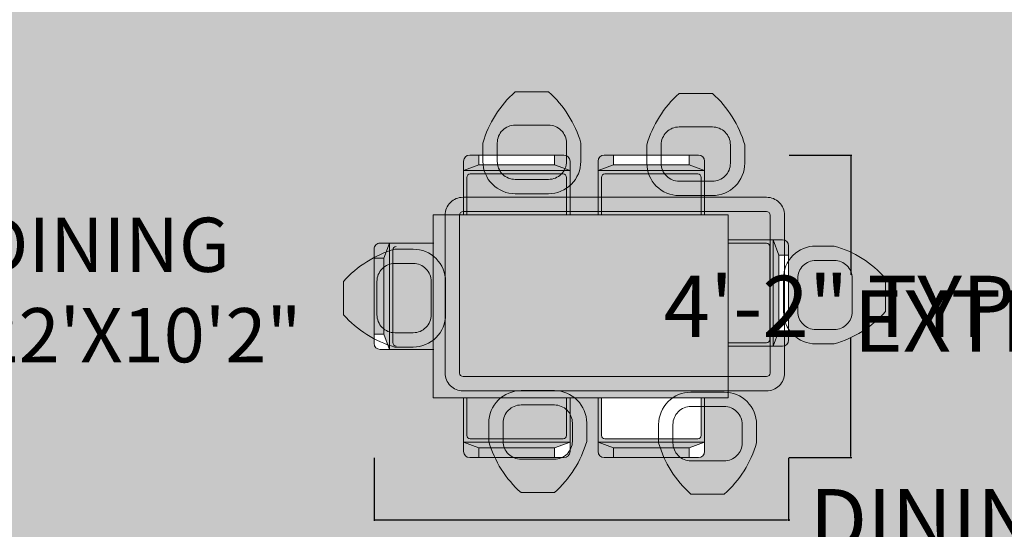
# Model space of a CAD drawing. Units: inches. Extents: x 1077 to 2505, y 1892 to 2728.
# Tile 14 of 26: x 1306 to 1470, y 2338 to 2422. Entities that reach past the tile are written whole.
import ezdxf

# ---------------------------------------------------------------- set-up
doc = ezdxf.new("R2010")
doc.units = ezdxf.units.IN
doc.linetypes.add('ACAD_ISO02W100', pattern=[15, 12, -3])
doc.layers.get('Defpoints').update_dxf_attribs({"color": 220, "linetype": 'ACAD_ISO02W100'})
for name, color, linetype, lineweight in [('00 FURNITURE', 15, 'Continuous', 15), ('A-ANNO-DIMS', 2, 'Continuous', 18), ('A-AREA-IDEN', 7, 'Continuous', 18)]:
    doc.layers.add(name, color=color, linetype=linetype, lineweight=lineweight)
doc.layers.add('A-FLOR-PATT', color=254, linetype='Continuous', lineweight=9, true_color=0xd7ebd2)
doc.styles.get("Standard").update_dxf_attribs({"font": 'arial.ttf'})
doc.dimstyles.get("Standard").update_dxf_attribs({"dimtxt": 10.18, "dimasz": 0.18, "dimexe": 0.18, "dimexo": 0.0625, "dimgap": 0.09, "dimtad": 0, "dimtih": 1, "dimtoh": 1, "dimdec": 0, "dimzin": 0, "dimdsep": 46, "dimlunit": 3, "dimtxsty": 'Standard', "dimcen": 0.09, "dimadec": 0, "dimazin": 0, "dimtfac": 1, "dimtdec": 0, "dimtofl": 0, "dimtmove": 0, "dimatfit": 3, "dimfxl": 1, "dimtolj": 1, "dimtzin": 0, "dimarcsym": 0})

# ---------------------------------------------------------------- blocks, each defined once
blk = doc.blocks.new('DINING-SET-6-SEAT')
for p, q in [((14.85, 40.27), (14.85, 49.18)), ((15.87, 50.2), (31.49, 50.2)), ((32.51, 49.18), (32.51, 40.27)), ((37.18, 40.27), (37.18, 49.18)), ((38.2, 50.2), (53.82, 50.2)), ((54.83, 49.18), (54.83, 40.27)), ((17.38, 48.59), (14.85, 47.63)), ((14.85, 47.63), (32.51, 47.63)), ((17.38, 48.59), (29.95, 48.59)), ((29.95, 48.59), (32.51, 47.63)), ((39.7, 48.59), (37.18, 47.63)), ((37.18, 47.63), (54.83, 47.63)), ((39.7, 48.59), (52.28, 48.59)), ((52.28, 48.59), (54.83, 47.63)), ((15.41, 40.27), (15.41, 46.51)), ((15.97, 47.07), (31.38, 47.07)), ((31.94, 46.51), (31.94, 40.27)), ((37.74, 40.27), (37.74, 46.51)), ((38.3, 47.07), (53.71, 47.07)), ((54.27, 46.51), (54.27, 40.27)), ((58.75, 40.27), (9.82, 40.27)), ((9.82, 9.93), (9.82, 40.27)), ((58.75, 9.93), (58.75, 40.27)), ((58.86, 36.15), (67.76, 36.15)), ((67.17, 33.62), (66.22, 36.15)), ((66.22, 36.15), (66.22, 18.49)), ((0, 34.59), (0, 18.97)), ((9.93, 35.61), (1.02, 35.61)), ((1.62, 33.08), (2.57, 35.61)), ((2.57, 35.61), (2.57, 17.96)), ((3.13, 34.49), (3.13, 19.08)), ((58.86, 35.58), (65.09, 35.58)), ((65.65, 35.02), (65.65, 19.61)), ((68.78, 35.13), (68.78, 19.51)), ((1.62, 33.08), (1.62, 20.51)), ((67.17, 33.62), (67.17, 21.04)), ((1.62, 20.51), (2.57, 17.96)), ((67.17, 21.04), (66.22, 18.49)), ((65.09, 19.05), (58.86, 19.05)), ((67.76, 18.49), (58.86, 18.49)), ((1.02, 17.96), (9.93, 17.96)), ((58.75, 9.93), (9.82, 9.93)), ((14.85, 9.93), (14.85, 1.02)), ((15.41, 9.93), (15.41, 3.69)), ((31.94, 3.69), (31.94, 9.93)), ((32.51, 1.02), (32.51, 9.93)), ((37.18, 9.93), (37.18, 1.02)), ((37.74, 9.93), (37.74, 3.69)), ((54.27, 3.69), (54.27, 9.93)), ((54.83, 1.02), (54.83, 9.93)), ((17.38, 1.61), (14.85, 2.57)), ((14.85, 2.57), (32.51, 2.57)), ((15.97, 3.13), (31.38, 3.13)), ((29.95, 1.61), (32.51, 2.57)), ((39.7, 1.61), (37.18, 2.57)), ((37.18, 2.57), (54.83, 2.57)), ((38.3, 3.13), (53.71, 3.13)), ((52.28, 1.61), (54.83, 2.57)), ((17.38, 1.61), (29.95, 1.61)), ((39.7, 1.61), (52.28, 1.61)), ((15.87, 0), (31.49, 0)), ((38.2, 0), (53.82, 0))]:
    blk.add_line(p, q)
for points in [[(17.38, 50.2), (29.95, 50.2), (29.95, 48.59), (17.38, 48.59)], [(39.7, 50.2), (52.28, 50.2), (52.28, 48.59), (39.7, 48.59)], [(0, 33.08), (0, 20.51), (1.62, 20.51), (1.62, 33.08)], [(68.78, 33.62), (68.78, 21.04), (67.17, 21.04), (67.17, 33.62)], [(17.38, 0), (29.95, 0), (29.95, 1.61), (17.38, 1.61)], [(39.7, 0), (52.28, 0), (52.28, 1.61), (39.7, 1.61)]]:
    blk.add_lwpolyline(points, close=True)
for centre, radius, start, end in [((15.87, 49.18), 1.02, 90.0001, 180.0001), ((31.49, 49.18), 1.02, 0.0001, 90.0001), ((38.2, 49.18), 1.02, 90.0001, 180.0001), ((53.82, 49.18), 1.02, 0.0001, 90.0001), ((15.97, 46.51), 0.56, 90.0001, 180.0001), ((31.38, 46.51), 0.56, 0.0001, 90.0001), ((38.3, 46.51), 0.56, 90.0001, 180.0001), ((53.71, 46.51), 0.56, 0.0001, 90.0001), ((67.76, 35.13), 1.02, 0.0001, 90.0001), ((1.02, 34.59), 1.02, 89.9999, 179.9999), ((3.69, 34.49), 0.56, 89.9999, 179.9999), ((65.09, 35.02), 0.56, 0.0001, 90.0001), ((65.09, 19.61), 0.56, 270.0001, 0.0001), ((1.02, 18.97), 1.02, 179.9999, 269.9999), ((3.69, 19.08), 0.56, 179.9999, 269.9999), ((67.76, 19.51), 1.02, 270.0001, 0.0001), ((15.97, 3.69), 0.56, 179.9999, 269.9999), ((31.38, 3.69), 0.56, 269.9999, 359.9999), ((38.3, 3.69), 0.56, 179.9999, 269.9999), ((53.71, 3.69), 0.56, 269.9999, 359.9999), ((15.87, 1.02), 1.02, 179.9999, 269.9999), ((31.49, 1.02), 1.02, 269.9999, 359.9999), ((38.2, 1.02), 1.02, 179.9999, 269.9999), ((53.82, 1.02), 1.02, 269.9999, 359.9999)]:
    blk.add_arc(centre, radius, start, end)
blk = doc.blocks.new('DINING-CHAIR')
for points in [[(5.36, 16.93), (10.88, 16.93, -0.142909), (16.24, 8.42), (16.24, 5.36, -0.414214), (10.88, 0), (5.36, 0, -0.414214), (0, 5.36), (0, 8.42, -0.142909)], [(5.36, 11.39), (10.88, 11.39, -0.414214), (13.86, 8.42), (13.86, 5.36, -0.414214), (10.88, 2.38), (5.36, 2.38, -0.414214), (2.38, 5.36), (2.38, 8.42, -0.414214)]]:
    blk.add_lwpolyline(points, format="xyb", close=True)
blk = doc.blocks.new('*D36')
at = {"layer": 'A-ANNO-DIMS', "color": 0, "lineweight": -2, "transparency": 16777216}
for p, q in [((1365.09, 2349.48), (1365.09, 2339.05)), ((1433.87, 2349.48), (1433.87, 2339.05)), ((1365.27, 2339.23), (1433.69, 2339.23)), ((1433.87, 2339.23), (1434.05, 2339.23))]:
    blk.add_line(p, q, dxfattribs=at)
at = {"layer": 'A-ANNO-DIMS', "color": 0, "transparency": 16777216}
for points in [[(1365.27, 2339.26), (1365.27, 2339.2), (1365.09, 2339.23)], [(1433.69, 2339.26), (1433.69, 2339.2), (1433.87, 2339.23)]]:
    blk.add_solid(points, dxfattribs=at)
at = {"layer": 'Defpoints', "color": 0, "transparency": 16777216}
for p in [(1365.09, 2349.54), (1433.87, 2349.54), (1433.87, 2339.23)]:
    blk.add_point(p, dxfattribs=at)
at = {"layer": 'A-ANNO-DIMS', "color": 0, "transparency": 16777216, "insert": (1507.58, 2339.23), "char_height": 10.18, "attachment_point": 5}
blk.add_mtext('\\A1;DINING SET 5\'-9" TYP.', dxfattribs=at)
blk = doc.blocks.new('*D37')
at = {"layer": 'A-ANNO-DIMS', "color": 0, "lineweight": -2, "transparency": 16777216}
for p, q in [((1433.94, 2399.74), (1444.37, 2399.74)), ((1444.19, 2399.56), (1444.19, 2379.85)), ((1444.19, 2349.72), (1444.19, 2369.44)), ((1433.94, 2349.54), (1444.37, 2349.54))]:
    blk.add_line(p, q, dxfattribs=at)
at = {"layer": 'A-ANNO-DIMS', "color": 0, "transparency": 16777216}
for points in [[(1444.16, 2399.56), (1444.22, 2399.56), (1444.19, 2399.74)], [(1444.16, 2349.72), (1444.22, 2349.72), (1444.19, 2349.54)]]:
    blk.add_solid(points, dxfattribs=at)
at = {"layer": 'Defpoints', "color": 0, "transparency": 16777216}
for p in [(1433.87, 2399.74), (1444.19, 2399.74), (1433.87, 2349.54)]:
    blk.add_point(p, dxfattribs=at)
at = {"layer": 'A-ANNO-DIMS', "color": 0, "transparency": 16777216, "insert": (1444.19, 2374.64), "char_height": 10.18, "attachment_point": 5}
blk.add_mtext('\\A1;4\'-2" TYP.', dxfattribs=at)
blk = doc.blocks.new('*D58')
at = {"layer": 'A-ANNO-DIMS', "color": 0, "lineweight": -2, "transparency": 16777216}
for p, q in [((1547.47, 2396.22), (1540.15, 2396.22)), ((1540.33, 2396.04), (1540.33, 2377.58)), ((1540.33, 2348.4), (1540.33, 2366.87)), ((1547.47, 2348.22), (1540.15, 2348.22))]:
    blk.add_line(p, q, dxfattribs=at)
at = {"layer": 'A-ANNO-DIMS', "color": 0, "transparency": 16777216}
for points in [[(1540.3, 2396.04), (1540.36, 2396.04), (1540.33, 2396.22)], [(1540.3, 2348.4), (1540.36, 2348.4), (1540.33, 2348.22)]]:
    blk.add_solid(points, dxfattribs=at)
at = {"layer": 'Defpoints', "color": 0, "transparency": 16777216}
for p in [(1547.53, 2396.22), (1540.33, 2348.22), (1547.53, 2348.22)]:
    blk.add_point(p, dxfattribs=at)
at = {"layer": 'A-ANNO-DIMS', "color": 0, "transparency": 16777216, "insert": (1540.33, 2372.22), "char_height": 10.18, "attachment_point": 5}
blk.add_mtext('\\A1;EXTERIOR WINDOW 4\'-0" TYP.', dxfattribs=at)

msp = doc.modelspace()

# ---------------------------------------------------------------- hatches: boundary and pattern name
at = {"layer": 'A-FLOR-PATT', "transparency": 33554559}
h = msp.add_hatch(color=256, dxfattribs=at)
h.dxf.hatch_style = 1
h.paths.add_polyline_path([(1395.53, 2577.16), (1374.83, 2577.16), (1350.83, 2577.19), (1350.83, 2577.16), (1329.53, 2577.16), (1329.53, 2480.16), (1329.53, 2469.16), (1325.53, 2469.16), (1325.53, 2515.13), (1307.53, 2515.13), (1307.53, 2577.16), (1269.31, 2577.16), (1221.31, 2577.15), (1221.31, 2577.16), (1187.53, 2577.16), (1187.53, 2433.16), (1289.53, 2433.16), (1289.53, 2429.16), (1263.53, 2429.16), (1187.53, 2429.16), (1187.53, 2395.02), (1187.53, 2395.02), (1187.53, 2371.02), (1187.53, 2371.02), (1187.53, 2307.16), (1259.53, 2307.16), (1259.53, 2399.16), (1263.53, 2399.16), (1263.53, 2307.16), (1289.53, 2307.16), (1289.53, 2306.23), (1325.53, 2306.23), (1325.53, 2307.16), (1329.53, 2307.16), (1329.53, 2306.23), (1365.53, 2306.23), (1365.53, 2307.16), (1432.53, 2307.16), (1432.53, 2088.16), (1547.53, 2088.16), (1547.53, 2140.08), (1511.53, 2140.08), (1511.53, 2267.16), (1475.53, 2267.16), (1475.53, 2303.16), (1468.53, 2303.16), (1468.53, 2307.16), (1547.53, 2307.16), (1547.53, 2348.22), (1547.53, 2396.22), (1547.53, 2429.16), (1435.53, 2429.16), (1435.53, 2433.16), (1476.35, 2433.16), (1476.35, 2451.18), (1547.53, 2451.18), (1547.53, 2577.16), (1499.53, 2577.16), (1499.53, 2586.16), (1547.53, 2586.16), (1547.53, 2642.16), (1518.18, 2642.16), (1518.18, 2642.05), (1494.15, 2642.05), (1494.15, 2642.16), (1469.53, 2642.16), (1469.53, 2577.16), (1399.53, 2577.16), (1399.53, 2429.16), (1325.53, 2429.16), (1325.53, 2433.16), (1329.53, 2433.16), (1395.53, 2433.16), (1395.53, 2480.16), (1359.53, 2480.16), (1359.53, 2484.16), (1395.53, 2484.16)])
h.paths.add_polyline_path([(1357.65, 2482.07), (1355.65, 2482.07), (1355.65, 2481.07, 0.414214), (1356.65, 2480.07), (1344.65, 2480.07), (1344.65, 2477.06), (1343.27, 2477.06), (1343.27, 2480.07), (1330.65, 2480.07, -0.414214), (1329.65, 2481.07), (1329.65, 2484.07), (1331.65, 2484.07), (1331.65, 2510.07, -0.446908)], flags=16)
h.paths.add_polyline_path([(1305.09, 2559.18), (1288.89, 2559.18), (1288.89, 2575.38), (1305.09, 2575.38)], flags=16)
h.paths.add_polyline_path([(1304.19, 2560.08), (1289.79, 2560.08), (1289.79, 2574.48), (1304.19, 2574.48)], flags=0)
h.paths.add_polyline_path([(1287.99, 2500.68, -0.414214), (1287.09, 2499.78), (1265.14, 2499.78), (1224.09, 2499.78, -0.414214), (1223.19, 2500.68), (1223.19, 2557.16), (1223.19, 2571.74), (1223.19, 2575.38), (1287.99, 2575.38), (1287.99, 2571.74), (1287.09, 2571.74, -0.414214), (1287.99, 2570.84)], flags=16)
h.paths.add_polyline_path([(1292.98, 2569.05, -1), (1300.92, 2569.05, -1)], flags=0)
h.paths.add_polyline_path([(1293.32, 2569.05, -1), (1300.58, 2569.05, -1)], flags=0)
h.paths.add_polyline_path([(1322.8, 2462.21), (1322.8, 2431.71), (1323.05, 2430.71), (1323.05, 2431.71), (1321.8, 2431.71), (1321.8, 2462.19, 0.404641), (1292.3, 2431.71), (1292.05, 2430.71, -0.414214), (1291.55, 2430.21), (1291.05, 2430.21), (1291.05, 2429.71, -0.414214), (1290.55, 2429.21), (1289.55, 2429.21), (1289.55, 2434.21), (1290.55, 2434.21, -0.414214), (1291.05, 2433.71), (1291.05, 2433.21), (1291.55, 2433.21, -0.414214), (1292.05, 2432.71), (1292.3, 2431.71, -0.414214)], flags=16)
h.paths.add_polyline_path([(1287.82, 2548.28, 0.292232), (1279.17, 2536.8, 0.052719), (1223.93, 2548.28), (1223.28, 2548.28), (1223.28, 2557.16), (1223.93, 2557.16), (1245.42, 2557.16, -0.117785), (1245.77, 2557.93, -0.059418), (1254.87, 2567.02, -0.379859), (1257.28, 2566.88, -0.02509), (1261.41, 2563.32, -0.025935), (1265.65, 2567.02, -0.379859), (1268.06, 2566.88, -0.061767), (1277.52, 2557.43, -0.069393), (1277.82, 2557.16), (1287.82, 2557.16)], flags=0)
h.paths.add_polyline_path([(1263.47, 2548.28), (1260.56, 2548.28, -0.015371), (1258.01, 2546.13, -0.429576), (1255.37, 2546.06, -0.016036), (1252.69, 2548.28), (1223.28, 2548.28), (1223.28, 2554.42), (1246.78, 2554.42, 0.055344), (1255.37, 2546.06, 0.331768), (1257.52, 2545.74, 0.027343), (1262, 2549.64, 0.00919)], flags=0)
h.paths.add_polyline_path([(1295.56, 2568.34), (1296.87, 2569.09), (1296.87, 2570.6, 0.399698), (1295.39, 2569.05, 0.119004)], flags=0)
h.paths.add_polyline_path([(1295.21, 2569.05, -1), (1298.68, 2569.05, -1)], flags=0)
h.paths.add_polyline_path([(1296.95, 2568.96), (1297.03, 2569), (1297.03, 2569.09), (1296.99, 2569.11), (1296.91, 2568.98)], flags=0)
h.paths.add_polyline_path([(1402.28, 2462.19, -0.414214), (1432.78, 2431.69), (1433.03, 2432.69), (1432.78, 2431.69, 0.404641), (1403.28, 2462.17), (1403.28, 2431.69), (1402.03, 2431.69), (1402.03, 2430.69, -0.414214), (1401.53, 2430.19), (1401.03, 2430.19), (1401.03, 2429.69, -0.414214), (1400.53, 2429.19), (1399.53, 2429.19), (1399.53, 2434.19), (1400.53, 2434.19, -0.414214), (1401.03, 2433.69), (1401.03, 2433.19), (1401.53, 2433.19, -0.414214), (1402.03, 2432.69)], flags=16)
h.paths.add_polyline_path([(1470.16, 2535.21, -0.414214), (1471.06, 2536.11), (1527.54, 2536.11), (1542.12, 2536.11), (1545.76, 2536.11), (1545.76, 2471.31), (1542.12, 2471.31), (1542.12, 2472.21, -0.414214), (1541.22, 2471.31), (1471.06, 2471.31, -0.414214), (1470.16, 2472.21), (1470.16, 2494.16)], flags=16)
h.paths.add_polyline_path([(1483.07, 2536.11, 0.253465), (1480.11, 2526.15, 0.2538), (1470.15, 2523.19)], flags=16)
h.paths.add_polyline_path([(1223.19, 2512.69, 0.253465), (1233.14, 2509.74, 0.2538), (1236.1, 2499.77)], flags=16)
h.paths.add_polyline_path([(1469.77, 2578.72), (1469.77, 2581.72), (1471.77, 2581.72), (1471.77, 2607.72, -0.01951), (1473.77, 2607.68), (1473.77, 2579.72), (1473.77, 2578.72, -0.414214), (1472.77, 2577.72), (1470.77, 2577.72, -0.414214)], flags=16)
h.paths.add_polyline_path([(1382.46, 2398.13), (1395.04, 2398.13), (1395.04, 2399.74), (1382.46, 2399.74)], flags=16)
h.paths.add_polyline_path([(1379.94, 2397.18), (1379.94, 2389.82), (1380.5, 2389.82), (1380.5, 2396.05, -0.41429), (1381.06, 2396.61), (1396.47, 2396.61, -0.414213), (1397.03, 2396.05), (1397.03, 2389.82), (1397.59, 2389.82), (1397.59, 2397.18)], flags=16)
h.paths.add_polyline_path([(1263.37, 2428.14), (1263.37, 2426.14, -0.414214), (1262.37, 2425.14), (1261.37, 2425.14), (1233.41, 2425.14, 0.400854), (1259.37, 2401.04), (1259.37, 2401.14), (1261.37, 2401.14, -0.446908), (1233.37, 2427.14), (1259.37, 2427.14), (1259.37, 2429.14), (1262.37, 2429.14, -0.414214)], flags=16)
h.paths.add_polyline_path([(1404.79, 2398.13), (1417.37, 2398.13), (1417.37, 2399.74), (1404.79, 2399.74)], flags=16)
h.paths.add_polyline_path([(1402.27, 2397.18), (1404.79, 2398.13), (1417.37, 2398.13), (1419.92, 2397.18)], flags=16)
h.paths.add_polyline_path([(1432.26, 2383.16), (1432.26, 2370.59), (1433.87, 2370.59), (1433.87, 2383.16)], flags=16)
h.paths.add_polyline_path([(1431.3, 2385.69), (1423.84, 2385.69), (1423.84, 2385.13), (1430.18, 2385.13, -0.41429), (1430.74, 2384.57), (1430.74, 2369.16, -0.414237), (1430.18, 2368.6), (1423.84, 2368.6), (1423.84, 2368.03), (1431.3, 2368.03)], flags=16)
h.paths.add_polyline_path([(1417.37, 2351.16), (1417.37, 2349.54), (1418.9, 2349.54, 0.414236), (1419.92, 2350.56), (1419.92, 2352.11)], flags=16)
h.paths.add_polyline_path([(1395.04, 2351.16), (1395.04, 2349.54), (1396.58, 2349.54, 0.414235), (1397.59, 2350.56), (1397.59, 2352.11)], flags=16)
h.paths.add_polyline_path([(1366.7, 2370.05), (1365.09, 2370.05), (1365.09, 2368.52, 0.414235), (1366.11, 2367.5), (1367.66, 2367.5)], flags=16)
h.paths.add_polyline_path([(1419.36, 2359.47), (1419.36, 2353.24, -0.41419), (1418.8, 2352.68), (1403.39, 2352.68, -0.414137), (1402.83, 2353.24), (1402.83, 2359.47), (1397.03, 2359.47), (1397.03, 2353.24, -0.414189), (1396.47, 2352.68), (1381.06, 2352.68, -0.414137), (1380.5, 2353.24), (1380.5, 2359.47)], flags=16)
h.paths.add_polyline_path([(1222.29, 2559.18), (1206.09, 2559.18), (1206.09, 2575.38), (1222.29, 2575.38)], flags=16)
h.paths.add_polyline_path([(1221.39, 2560.08), (1206.99, 2560.08), (1206.99, 2574.48), (1221.39, 2574.48)], flags=0)
h.paths.add_polyline_path([(1482, 2577.72), (1482, 2580.73), (1483.38, 2580.73), (1483.38, 2577.72), (1484.77, 2577.72), (1484.77, 2574.72), (1483.38, 2574.72), (1483.38, 2577.72)], flags=16)
h.paths.add_polyline_path([(1266.37, 2415.53), (1266.37, 2414.14), (1263.37, 2414.14), (1263.37, 2415.53), (1260.36, 2415.53), (1260.36, 2416.91), (1263.37, 2416.91), (1263.37, 2415.53)], flags=16)
h.paths.add_polyline_path([(1210.26, 2569.05, -1), (1218.19, 2569.05, -1)], flags=0)
h.paths.add_polyline_path([(1210.6, 2569.05, -1), (1217.85, 2569.05, -1)], flags=0)
h.paths.add_polyline_path([(1212.84, 2568.34), (1214.15, 2569.09), (1214.15, 2570.6, 0.399698), (1212.67, 2569.05, 0.119004)], flags=0)
h.paths.add_polyline_path([(1212.49, 2569.05, -1), (1215.96, 2569.05, -1)], flags=0)
h.paths.add_polyline_path([(1214.23, 2568.96), (1214.3, 2568.91), (1214.3, 2569)], flags=0)
h.paths.add_polyline_path([(1507.18, 2480.12, 0.052719), (1518.66, 2535.36), (1518.66, 2536.01), (1527.54, 2536.01), (1527.54, 2535.36), (1527.54, 2513.88, -0.117785), (1528.31, 2513.53, -0.059418), (1537.4, 2504.43, -0.379859), (1537.26, 2502.01, -0.02509), (1533.7, 2497.89, -0.025935), (1537.4, 2493.64, -0.379859), (1537.26, 2491.23, -0.061767), (1527.8, 2481.77, -0.069393), (1527.54, 2481.47), (1527.54, 2471.47), (1518.66, 2471.47, 0.292232)], flags=0)
h.paths.add_polyline_path([(1516.43, 2503.92, -0.016036), (1518.66, 2506.6), (1518.66, 2536.01), (1524.8, 2536.01), (1524.8, 2512.51, 0.055344), (1516.43, 2503.92, 0.331768), (1516.12, 2501.77, 0.027343), (1520.01, 2497.29, 0.00919), (1518.66, 2495.82), (1518.66, 2498.73, -0.015371), (1516.5, 2501.28, -0.429576)], flags=0)
h.paths.add_polyline_path([(1499.63, 2625.5, -0.171636), (1502.82, 2631.01), (1502.82, 2633.37), (1498.68, 2633.37, -0.414214), (1497.7, 2634.36), (1497.7, 2640.66, -0.414214), (1498.68, 2641.64), (1514.82, 2641.64, -0.414214), (1515.81, 2640.66), (1515.81, 2634.36, -0.414214), (1514.82, 2633.37), (1510.69, 2633.37), (1510.69, 2631.01, -0.171636), (1513.88, 2625.5, -0.258205), (1509.31, 2614.47), (1504.19, 2614.47, -0.258205)], flags=16)
h.paths.add_polyline_path([(1501.2, 2625.5, -0.171636), (1504.39, 2631.01), (1509.12, 2631.01, -0.171636), (1512.3, 2625.5, -0.210384), (1509.35, 2616.02), (1504.16, 2616.02, -0.210384)], flags=0)
h.paths.add_polyline_path([(1529.56, 2537.01), (1529.56, 2553.21), (1545.76, 2553.21), (1545.76, 2537.01)], flags=16)
h.paths.add_polyline_path([(1530.46, 2537.91), (1530.46, 2552.31), (1544.86, 2552.31), (1544.86, 2537.91)], flags=0)
h.paths.add_polyline_path([(1535.45, 2545.07, -1), (1543.39, 2545.07, -1)], flags=0)
h.paths.add_polyline_path([(1535.8, 2545.07, -1), (1543.05, 2545.07, -1)], flags=0)
h.paths.add_polyline_path([(1529.56, 2470.41), (1545.76, 2470.41), (1545.76, 2454.21), (1529.56, 2454.21)], flags=16)
h.paths.add_polyline_path([(1541.16, 2544.99), (1540.98, 2544.99, -0.544606), (1538.71, 2543.68), (1538.62, 2543.53, 0.547962)], flags=0)
h.paths.add_polyline_path([(1530.46, 2469.51), (1544.86, 2469.51), (1544.86, 2455.11), (1530.46, 2455.11)], flags=0)
h.paths.add_polyline_path([(1539.47, 2545.14), (1539.42, 2545.22), (1539.38, 2545.14)], flags=0)
h.paths.add_polyline_path([(1543.39, 2462.34, -1), (1535.45, 2462.34, -1)], flags=0)
h.paths.add_polyline_path([(1543.05, 2462.34, -1), (1535.8, 2462.34, -1)], flags=0)
h.paths.add_polyline_path([(1541.16, 2462.27), (1540.98, 2462.27, -0.544606), (1538.71, 2460.96), (1538.62, 2460.8, 0.547962)], flags=0)
h.paths.add_polyline_path([(1539.47, 2462.42), (1539.42, 2462.5), (1539.38, 2462.42)], flags=0)
h.paths.add_polyline_path([(1435.32, 2335.25, -0.414214), (1465.82, 2304.75), (1466.07, 2305.75), (1465.82, 2304.75, 0.404641), (1436.32, 2335.23), (1436.32, 2304.75), (1435.07, 2304.75), (1435.07, 2303.75, -0.414214), (1434.57, 2303.25), (1434.07, 2303.25), (1434.07, 2302.75, -0.414214), (1433.57, 2302.25), (1432.57, 2302.25), (1432.57, 2307.25), (1433.57, 2307.25, -0.414214), (1434.07, 2306.75), (1434.07, 2306.25), (1434.57, 2306.25, -0.414214), (1435.07, 2305.75)], flags=16)
h.paths.add_polyline_path([(1532.13, 2635.71), (1535.43, 2635.71), (1535.43, 2635.89), (1532.13, 2635.89)], flags=16)
edge = h.paths.add_edge_path(flags=16)
edge.add_arc((1535.98, 2632.67), 0.183, 270, 360)
edge.add_line((1536.17, 2632.67), (1536.17, 2639.82))
edge.add_line((1536.17, 2639.82), (1538.29, 2639.82))
edge.add_line((1538.29, 2639.82), (1538.29, 2641.82))
edge.add_line((1538.29, 2641.82), (1533.25, 2641.82))
edge.add_line((1533.25, 2641.82), (1533.25, 2639.82))
edge.add_line((1533.25, 2639.82), (1534.87, 2639.82))
edge.add_line((1534.87, 2639.82), (1534.87, 2639))
edge.add_line((1534.87, 2639), (1533.7, 2639))
edge.add_line((1533.7, 2639), (1533.7, 2639.82))
edge.add_line((1533.7, 2639.82), (1533.25, 2639.82))
edge.add_line((1533.25, 2639.82), (1533.25, 2641.82))
edge.add_line((1533.25, 2641.82), (1538.29, 2641.82))
edge.add_line((1538.29, 2641.82), (1538.29, 2641.34))
edge.add_line((1538.29, 2641.34), (1540.64, 2641.58))
edge.add_line((1540.64, 2641.58), (1540.64, 2641.82))
edge.add_line((1540.64, 2641.82), (1541.5, 2641.82))
edge.add_line((1541.5, 2641.82), (1541.5, 2641.25))
edge.add_line((1541.5, 2641.25), (1541.31, 2639.79))
edge.add_ellipse((1541.09, 2638.95), major_axis=(-1.08, 0), ratio=0.790849, start_angle=180, end_angle=255.2976, ccw=False)
edge.add_line((1542.17, 2638.95), (1542.17, 2638.38))
edge.add_ellipse((1541.09, 2638.38), major_axis=(-1.08, 0), ratio=0.790849, start_angle=0, end_angle=180, ccw=False)
edge.add_line((1540, 2638.38), (1540.01, 2638.87))
edge.add_ellipse((1541.09, 2638.95), major_axis=(-1.08, 0), ratio=0.790849, start_angle=284.7024, end_angle=364.0401, ccw=False)
edge.add_line((1540.78, 2639.75), (1540.78, 2641.25))
edge.add_line((1540.78, 2641.25), (1540.64, 2641.25))
edge.add_line((1540.64, 2641.25), (1538.29, 2641.01))
edge.add_line((1538.29, 2641.01), (1538.29, 2639.82))
edge.add_line((1538.29, 2639.82), (1536.17, 2639.82))
edge.add_line((1536.17, 2639.82), (1536.17, 2632.48))
edge.add_line((1536.17, 2632.48), (1535.98, 2632.48))
h.paths.add_polyline_path([(1496.32, 2250.34, -0.292371), (1498.9, 2247.83, -0.085148), (1501.21, 2208.85, -0.01331), (1500.27, 2098.5, -0.379287), (1497.22, 2095.28, -0.0502), (1441.54, 2095.28, -0.379287), (1438.5, 2098.5, -0.01331), (1437.56, 2208.85, -0.086132), (1439.96, 2248.26, -0.295116), (1442.59, 2250.78, -0.114238)], flags=16)
h.paths.add_polyline_path([(1495.16, 2205.84, -0.355389), (1496.7, 2202.1), (1492.94, 2189.65, -0.398275), (1489.12, 2187.47, 0.113332), (1449.64, 2187.47, -0.398275), (1445.82, 2189.65), (1442.06, 2202.1, -0.355394), (1443.6, 2205.84, -0.265725)], flags=0)
h.paths.add_polyline_path([(1440.37, 2195.72), (1445.94, 2181.67), (1445.94, 2160.63), (1440.84, 2157.26)], flags=0)
h.paths.add_polyline_path([(1498.46, 2195.72), (1497.99, 2157.26), (1492.88, 2160.63), (1492.88, 2181.67)], flags=0)
h.paths.add_polyline_path([(1445.94, 2158.37), (1445.94, 2137.12), (1441.12, 2122.56), (1440.87, 2155.03)], flags=0)
h.paths.add_polyline_path([(1492.88, 2158.37), (1497.96, 2155.03), (1497.71, 2122.56), (1492.88, 2137.12)], flags=0)
h.paths.add_polyline_path([(1489.88, 2130.4), (1494.39, 2107.67, -0.090102), (1444.44, 2107.65), (1448.95, 2130.39, 0.036636)], flags=0)
h.paths.add_polyline_path([(1447.54, 2159.34), (1497.44, 2159.34), (1497.44, 2177.89), (1447.54, 2177.89)], flags=8)
h.paths.add_polyline_path([(1196.44, 2354.84), (1246.65, 2354.84), (1246.65, 2388.43), (1196.44, 2388.43)], flags=24)
h.paths.add_polyline_path([(1296.09, 2360.25), (1353.81, 2360.25), (1353.81, 2393.84), (1296.09, 2393.84)], flags=24)
h.paths.add_polyline_path([(1400.72, 2471.85), (1470.63, 2471.85), (1470.63, 2505.44), (1400.72, 2505.44)], flags=24)
h.paths.add_polyline_path([(1324.78, 2448.48), (1394.95, 2448.48), (1394.95, 2467.02), (1324.78, 2467.02)], flags=24)
h.paths.add_polyline_path([(1335.08, 2531.43), (1389.67, 2531.43), (1389.67, 2565.02), (1335.08, 2565.02)], flags=24)
h.paths.add_polyline_path([(1225.76, 2460), (1295.67, 2460), (1295.67, 2493.58), (1225.76, 2493.58)], flags=24)
h = msp.add_hatch(color=256, dxfattribs=at)
h.dxf.hatch_style = 1
h.paths.add_polyline_path([(1547.53, 2348.22), (1547.53, 2396.22), (1547.53, 2425.11), (1547.53, 2425.11), (1547.53, 2429.16), (1435.53, 2429.16), (1434.03, 2429.21), (1434.03, 2430.19), (1433.03, 2430.19), (1432.78, 2431.69, 0.404641), (1403.28, 2462.17), (1403.28, 2431.69), (1402.03, 2431.69), (1402.03, 2430.19), (1401.03, 2430.19), (1401.03, 2429.19), (1399.53, 2429.19), (1399.53, 2429.19), (1399.53, 2429.16), (1334.67, 2429.16), (1334.67, 2423.95), (1325.67, 2423.95), (1325.67, 2429.16), (1325.53, 2429.16), (1324.05, 2429.24), (1324.05, 2430.21), (1323.05, 2430.21), (1323.05, 2431.71), (1321.8, 2431.71), (1321.8, 2462.19, 0.416544), (1292.05, 2430.73, -0.423614), (1291.55, 2430.21), (1291.05, 2430.21), (1291.05, 2429.21), (1289.55, 2429.21), (1289.53, 2429.21), (1289.53, 2429.16), (1263.37, 2429.16), (1263.37, 2415.53), (1266.37, 2415.53), (1266.37, 2414.14), (1263.37, 2414.14), (1263.37, 2399.16), (1263.53, 2399.16), (1263.53, 2307.16), (1289.53, 2307.16), (1289.53, 2306.23), (1323.26, 2306.23), (1323.26, 2307.21), (1332.26, 2307.21), (1365.53, 2306.23), (1365.53, 2307.16), (1432.53, 2307.16), (1432.57, 2307.16), (1432.57, 2307.25), (1434.07, 2307.25), (1434.07, 2306.25), (1435.32, 2306.25), (1435.32, 2335.25, -0.407346), (1466.07, 2305.73, -0.423614), (1466.57, 2306.25), (1467.07, 2306.25), (1467.07, 2307.25), (1468.57, 2307.25), (1547.53, 2307.16), (1547.53, 2307.2)])
h.paths.add_polyline_path([(1430.74, 2369.16), (1430.74, 2384.57, 0.41429), (1430.18, 2385.13), (1423.84, 2385.13), (1423.84, 2368.6), (1430.18, 2368.6, 0.414237)], flags=16)
h.paths.add_polyline_path([(1432.26, 2383.16), (1432.26, 2370.59), (1433.87, 2370.59), (1433.87, 2383.16)], flags=16)
h.paths.add_polyline_path([(1431.3, 2368.03), (1431.3, 2385.69), (1432.26, 2383.16), (1432.26, 2370.59)], flags=16)
h.paths.add_polyline_path([(1417.37, 2351.16), (1417.37, 2349.54), (1418.9, 2349.54, 0.414236), (1419.92, 2350.56), (1419.92, 2352.11)], flags=16)
h.paths.add_polyline_path([(1403.39, 2352.68), (1418.78, 2352.68, 0.42427), (1419.36, 2353.24), (1419.36, 2359.47), (1402.83, 2359.47), (1402.83, 2353.24, 0.414137)], flags=16)
h.paths.add_polyline_path([(1366.7, 2370.05), (1365.09, 2370.05), (1365.09, 2368.52, 0.414235), (1366.11, 2367.5), (1367.66, 2367.5)], flags=16)
h.paths.add_polyline_path([(1382.46, 2398.13), (1395.04, 2398.13), (1395.04, 2399.74), (1382.46, 2399.74)], flags=16)
h.paths.add_polyline_path([(1396.47, 2396.61), (1381.06, 2396.61, 0.41429), (1380.5, 2396.05), (1380.5, 2389.82), (1397.03, 2389.82), (1397.03, 2396.05, 0.414213)], flags=16)
h.paths.add_polyline_path([(1402.27, 2397.18), (1402.83, 2396.05, -0.414213), (1403.39, 2396.61)], flags=16)
h.paths.add_polyline_path([(1418.8, 2396.61), (1419.36, 2396.61), (1419.36, 2396.05, 0.414237)], flags=16)
h.paths.add_polyline_path([(1404.79, 2398.13), (1417.37, 2398.13), (1417.37, 2399.74), (1404.79, 2399.74)], flags=16)
h.paths.add_polyline_path([(1381.06, 2352.68, -0.414213), (1380.5, 2353.24), (1380.27, 2352.11)], flags=16)
h.paths.add_polyline_path([(1396.58, 2349.54), (1396.58, 2349.54), (1395.04, 2349.54), (1395.04, 2349.54), (1382.46, 2349.54), (1382.46, 2351.16), (1395.04, 2351.16), (1397.59, 2352.11), (1397.59, 2350.56, -0.414235)], flags=16)
h.paths.add_polyline_path([(1379.94, 2397.18), (1382.46, 2398.13), (1395.04, 2398.13), (1397.59, 2397.18)], flags=16)
h.paths.add_polyline_path([(1368.78, 2384.59, 0.414213), (1368.22, 2384.03), (1367.66, 2367.5), (1367.66, 2385.15)], flags=16)
h.paths.add_polyline_path([(1547.53, 2574.38), (1547.51, 2574.38), (1547.51, 2577.16), (1499.53, 2577.16), (1484.77, 2577.44), (1484.77, 2574.72), (1483.38, 2574.72), (1483.38, 2577.72), (1482, 2577.72), (1469.53, 2577.72), (1469.53, 2577.16), (1401.95, 2577.16), (1401.95, 2574.12), (1399.53, 2574.12), (1399.53, 2434.19), (1401.03, 2434.19), (1401.03, 2433.19), (1402.28, 2433.19), (1402.28, 2462.19, -0.407346), (1433.03, 2432.67, -0.423614), (1433.53, 2433.19), (1434.03, 2433.19), (1434.03, 2434.19), (1435.53, 2434.19), (1476.35, 2433.81), (1476.35, 2451.18), (1547.53, 2451.18)])
h.paths.add_polyline_path([(1470.16, 2535.21, -0.414214), (1471.06, 2536.11), (1527.54, 2536.11), (1542.12, 2536.11), (1545.76, 2536.11), (1545.76, 2471.31), (1542.12, 2471.31), (1542.12, 2472.21, -0.414214), (1541.22, 2471.31), (1471.06, 2471.31, -0.414214), (1470.16, 2472.21), (1470.16, 2494.16)], flags=16)
h.paths.add_polyline_path([(1483.07, 2536.11, 0.253465), (1480.11, 2526.15, 0.2538), (1470.15, 2523.19)], flags=16)
h.paths.add_polyline_path([(1525.55, 2481.52, -0.000893), (1524.8, 2482.24), (1524.8, 2471.47), (1527.54, 2471.47), (1527.54, 2472.12), (1527.54, 2481.47, -0.388819)], flags=0)
h.paths.add_polyline_path([(1518.66, 2536.01), (1527.54, 2536.01), (1527.54, 2535.36), (1527.54, 2513.88, -0.117785), (1528.31, 2513.53, -0.059418), (1537.4, 2504.43, -0.379859), (1537.26, 2502.01, -0.02509), (1533.7, 2497.89, 0.033431), (1528.3, 2502.74, 0.308459), (1526.25, 2502.88, 0.047827), (1518.66, 2495.82), (1518.66, 2498.73, -0.015371), (1516.5, 2501.28, -0.429576), (1516.43, 2503.92, -0.016036), (1518.66, 2506.6)], flags=0)
h.paths.add_polyline_path([(1529.56, 2537.01), (1529.56, 2553.21), (1545.76, 2553.21), (1545.76, 2537.01)], flags=16)
h.paths.add_polyline_path([(1530.46, 2537.91), (1530.46, 2552.31), (1544.86, 2552.31), (1544.86, 2537.91)], flags=0)
h.paths.add_polyline_path([(1535.8, 2545.07, -1), (1543.05, 2545.07, -1)], flags=0)
h.paths.add_polyline_path([(1541.16, 2544.99), (1540.98, 2544.99, -0.544606), (1538.71, 2543.68), (1538.62, 2543.53, 0.547962)], flags=0)
h.paths.add_polyline_path([(1539.47, 2545.14), (1539.42, 2545.22), (1539.38, 2545.14)], flags=0)
h.paths.add_polyline_path([(1529.56, 2470.41), (1545.76, 2470.41), (1545.76, 2454.21), (1529.56, 2454.21)], flags=16)
h.paths.add_polyline_path([(1530.46, 2469.51), (1544.86, 2469.51), (1544.86, 2455.11), (1530.46, 2455.11)], flags=0)
h.paths.add_polyline_path([(1535.8, 2462.34, -1), (1543.05, 2462.34, -1)], flags=0)
h.paths.add_polyline_path([(1541.16, 2462.27), (1540.98, 2462.27, -0.544606), (1538.71, 2460.96), (1538.62, 2460.8, 0.547962)], flags=0)
h.paths.add_polyline_path([(1539.47, 2462.42), (1539.42, 2462.5), (1539.38, 2462.42)], flags=0)
h.paths.add_polyline_path([(1395.53, 2574.12), (1392.95, 2574.12), (1392.95, 2577.16), (1374.83, 2577.16), (1350.83, 2577.19), (1350.83, 2577.16), (1332.07, 2577.16), (1332.07, 2574), (1329.53, 2574), (1329.53, 2484.07), (1331.65, 2484.07), (1331.65, 2510.07, -0.423677), (1357.76, 2484.07), (1359.53, 2484.07), (1359.53, 2484.16), (1395.53, 2484.16)], flags=17)
h.paths.add_polyline_path([(1395.53, 2480.16), (1359.06, 2480.16, 0.437533), (1359.53, 2481.55), (1359.53, 2484.16), (1395.53, 2484.16), (1395.53, 2574.12), (1392.95, 2574.12), (1392.95, 2577.16), (1374.83, 2577.16), (1350.83, 2577.19), (1350.83, 2577.16), (1332.07, 2577.16), (1332.07, 2574), (1329.53, 2574), (1329.53, 2484.07), (1329.65, 2484.07), (1329.65, 2481.07), (1329.53, 2480.16), (1329.53, 2469.16), (1325.53, 2469.16), (1325.53, 2515.13), (1307.53, 2515.13), (1307.53, 2577.16), (1269.31, 2577.16), (1221.31, 2577.15), (1221.31, 2577.16), (1187.61, 2577.16), (1187.61, 2574.03), (1187.53, 2433.16), (1289.55, 2433.16), (1289.55, 2434.21), (1291.05, 2434.21), (1291.05, 2433.21), (1292.05, 2433.21), (1292.3, 2431.71, -0.414214), (1322.8, 2462.21), (1323.05, 2432.71, -0.414214), (1323.55, 2433.21), (1324.05, 2433.21), (1324.05, 2434.21), (1325.67, 2434.21), (1325.67, 2435.95), (1334.67, 2435.95), (1334.67, 2433.16), (1395.53, 2433.16)])
h.paths.add_polyline_path([(1344.65, 2480.07), (1344.65, 2477.06), (1343.27, 2477.06), (1343.27, 2480.07), (1332.65, 2480.07, 0.414214), (1333.65, 2481.07), (1333.65, 2482.07), (1331.65, 2482.07), (1331.65, 2484.07), (1331.65, 2510.07, -0.446908), (1357.65, 2482.07), (1355.65, 2482.07), (1355.65, 2481.07, 0.414214), (1356.65, 2480.07)], flags=16)
h.paths.add_polyline_path([(1287.99, 2500.68, -0.414214), (1287.09, 2499.78), (1265.14, 2499.78), (1224.09, 2499.78, -0.414214), (1223.19, 2500.68), (1223.19, 2557.16), (1223.19, 2571.74), (1223.19, 2575.38), (1287.99, 2575.38), (1287.99, 2571.74), (1287.09, 2571.74, -0.414214), (1287.99, 2570.84)], flags=16)
h.paths.add_polyline_path([(1277.77, 2555.17, -0.000893), (1277.05, 2554.42), (1287.82, 2554.42), (1287.82, 2557.16), (1287.17, 2557.16), (1277.82, 2557.16, -0.388819)], flags=0)
h.paths.add_polyline_path([(1223.28, 2548.28), (1223.28, 2557.16), (1223.93, 2557.16), (1245.42, 2557.16, -0.117785), (1245.77, 2557.93, -0.059418), (1254.87, 2567.02, -0.379859), (1257.28, 2566.88, -0.02509), (1261.41, 2563.32, 0.033431), (1256.55, 2557.93, 0.308459), (1256.41, 2555.88, 0.047827), (1263.47, 2548.28), (1260.56, 2548.28, -0.015371), (1258.01, 2546.13, -0.429576), (1255.37, 2546.06, -0.016036), (1252.69, 2548.28)], flags=0)
h.paths.add_polyline_path([(1305.09, 2559.18), (1288.89, 2559.18), (1288.89, 2575.38), (1305.09, 2575.38)], flags=16)
h.paths.add_polyline_path([(1304.19, 2560.08), (1289.79, 2560.08), (1289.79, 2574.48), (1304.19, 2574.48)], flags=0)
h.paths.add_polyline_path([(1300.58, 2569.05, -1), (1293.32, 2569.05, -1)], flags=0)
h.paths.add_polyline_path([(1223.19, 2512.69, 0.253465), (1233.14, 2509.74, 0.2538), (1236.1, 2499.77)], flags=16)
h.paths.add_polyline_path([(1295.56, 2568.34), (1296.87, 2569.09), (1296.87, 2570.6, 0.399698), (1295.39, 2569.05, 0.119004)], flags=0)
h.paths.add_polyline_path([(1295.21, 2569.05, -1), (1298.68, 2569.05, -1)], flags=0)
h.paths.add_polyline_path([(1296.95, 2568.96), (1297.03, 2569), (1297.03, 2569.09), (1296.99, 2569.11), (1296.91, 2568.98)], flags=0)
h.paths.add_polyline_path([(1222.29, 2559.18), (1206.09, 2559.18), (1206.09, 2575.38), (1222.29, 2575.38)], flags=16)
h.paths.add_polyline_path([(1221.39, 2560.08), (1206.99, 2560.08), (1206.99, 2574.48), (1221.39, 2574.48)], flags=0)
h.paths.add_polyline_path([(1217.85, 2569.05, -1), (1210.6, 2569.05, -1)], flags=0)
h.paths.add_polyline_path([(1212.84, 2568.34), (1214.15, 2569.09), (1214.15, 2570.6, 0.399698), (1212.67, 2569.05, 0.119004)], flags=0)
h.paths.add_polyline_path([(1212.49, 2569.05, -1), (1215.96, 2569.05, -1)], flags=0)
h.paths.add_polyline_path([(1214.23, 2568.96), (1214.3, 2569), (1214.3, 2569.09), (1214.26, 2569.11), (1214.19, 2568.98)], flags=0)
h.paths.add_polyline_path([(1259.53, 2399.14), (1259.37, 2399.14), (1259.37, 2401.04, -0.423677), (1233.37, 2427.14), (1259.37, 2427.14), (1259.37, 2429.16), (1187.53, 2429.16), (1187.53, 2395.02), (1187.53, 2395.02), (1187.53, 2371.02), (1187.53, 2371.02), (1187.53, 2311.49), (1187.55, 2311.49), (1187.55, 2307.16), (1259.53, 2307.16)])
h.paths.add_polyline_path([(1323.26, 2295.21), (1323.26, 2304.23), (1289.53, 2304.23), (1289.53, 2303.16), (1187.55, 2303.16), (1187.55, 2299.49), (1178.53, 2299.49), (1178.53, 2267.66), (1178.53, 2219.66), (1182.03, 2219.66), (1182.03, 2267.67), (1184.03, 2267.67), (1184.03, 2219.66), (1187.53, 2219.66), (1187.53, 2153.16), (1228.13, 2153.16), (1276.13, 2153.16), (1276.13, 2153.16), (1324.54, 2153.16), (1324.54, 2154.67), (1325.54, 2154.67), (1325.54, 2155.92), (1296.54, 2155.92, -0.407346), (1326.06, 2186.67, -0.423614), (1325.54, 2187.17), (1325.54, 2187.67), (1324.54, 2187.67), (1324.54, 2189.17), (1325.43, 2295.21)])
h.paths.add_polyline_path([(1432.53, 2307.16), (1365.53, 2307.16), (1365.53, 2306.23), (1365.53, 2303.16), (1428.53, 2303.16), (1428.53, 2221.2), (1428.57, 2221.2), (1428.57, 2197.2), (1428.53, 2197.16), (1428.53, 2303.01), (1404.46, 2303.01), (1404.46, 2221.2), (1329.53, 2221.2), (1329.53, 2307.16), (1325.53, 2307.16), (1325.53, 2295.21), (1325.43, 2295.21), (1324.54, 2189.17), (1324.54, 2187.67), (1326.04, 2187.67, 1.016365), (1326.06, 2186.67, 0.407348), (1296.54, 2155.92), (1325.54, 2155.92), (1325.54, 2154.67), (1324.54, 2154.67), (1324.54, 2153.16), (1329.53, 2153.16), (1329.53, 2144.16), (1432.53, 2144.16)])
h.paths.add_polyline_path([(1361.95, 2194.26), (1361.95, 2193.16), (1329.53, 2193.16), (1329.53, 2189.16), (1329.54, 2188.17), (1329.54, 2189.16), (1329.53, 2189.16), (1329.53, 2193.16), (1361.95, 2193.16), (1361.95, 2196.26), (1409.95, 2196.26), (1409.95, 2194.26)], flags=16)
h.paths.add_polyline_path([(1377.02, 2200.5), (1345.91, 2200.5), (1345.91, 2218.4), (1347.87, 2218.4), (1347.87, 2219.18), (1374.75, 2219.18), (1374.75, 2218.4), (1377.02, 2218.4)], flags=16)
h.paths.add_polyline_path([(1367.07, 2210.7, -1), (1373.34, 2210.7, -1)], flags=0)
h.paths.add_polyline_path([(1349.92, 2210.7, -1), (1356.98, 2210.7, -1)], flags=0)
h.paths.add_polyline_path([(1405.95, 2256.57), (1405.95, 2277.6), (1427.86, 2277.6), (1427.86, 2256.57)], flags=16)
h.paths.add_polyline_path([(1412.92, 2258.68, -0.414201), (1410.93, 2260.67), (1410.93, 2273.62, -0.414239), (1412.92, 2275.61), (1423.88, 2275.61, -0.414227), (1425.87, 2273.62), (1425.87, 2260.67, -0.414214), (1423.88, 2258.68)], flags=0)
h.paths.add_polyline_path([(1407.61, 2263.66, -1), (1409.18, 2263.66, -1)], flags=0)
h.paths.add_polyline_path([(1407.61, 2267.14, -1), (1409.18, 2267.14, -1)], flags=0)
h.paths.add_polyline_path([(1416.91, 2267.15, -1), (1419.89, 2267.15, -1)], flags=0)
h.paths.add_polyline_path([(1407.61, 2270.63, -1), (1409.18, 2270.63, -1)], flags=0)
h.paths.add_polyline_path([(1475.53, 2303.16), (1468.57, 2303.16), (1468.57, 2302.25), (1467.07, 2302.25), (1467.07, 2303.25), (1466.07, 2303.25), (1465.82, 2304.75, 0.404641), (1436.32, 2335.23), (1436.32, 2304.75), (1435.07, 2304.75), (1435.07, 2303.25), (1434.07, 2303.25), (1434.07, 2302.25), (1432.53, 2302.25), (1432.53, 2144.16), (1432.53, 2088.16), (1547.52, 2088.16), (1547.52, 2100.19), (1547.52, 2140.08), (1511.53, 2140.08), (1511.53, 2267.16), (1475.53, 2267.16)])
h.paths.add_polyline_path([(1438.35, 2102.86, 0.033498), (1438.37, 2102.21, -0.000079)], flags=16)
h.paths.add_polyline_path([(1496.32, 2250.34, -0.292371), (1498.9, 2247.83, -0.085148), (1501.21, 2208.85, -0.012784), (1500.42, 2102.86, -0.033498), (1500.39, 2102.21, 0.012863), (1501.21, 2208.85, 0.077283), (1499.67, 2244.3, 0.265882), (1497.48, 2246.8, 0.14401), (1441.46, 2247.36, 0.270646), (1439.21, 2244.85, -0.007564), (1439.96, 2248.26, -0.295116), (1442.59, 2250.78, -0.114238)], flags=16)
h.paths.add_polyline_path([(1495.16, 2205.84, -0.355389), (1496.7, 2202.1), (1492.94, 2189.65, -0.398275), (1489.12, 2187.47, 0.113332), (1449.64, 2187.47, -0.398275), (1445.82, 2189.65), (1442.06, 2202.1, -0.355394), (1443.6, 2205.84, -0.265725)], flags=16)
h.paths.add_polyline_path([(1440.37, 2195.72), (1445.94, 2181.67), (1445.94, 2160.63), (1440.84, 2157.26)], flags=16)
h.paths.add_polyline_path([(1498.46, 2195.72), (1497.99, 2157.26), (1492.88, 2160.63), (1492.88, 2181.67)], flags=16)
h.paths.add_polyline_path([(1445.94, 2158.37), (1445.94, 2137.12), (1441.12, 2122.56), (1440.87, 2155.03)], flags=16)
h.paths.add_polyline_path([(1492.88, 2158.37), (1497.96, 2155.03), (1497.71, 2122.56), (1492.88, 2137.12)], flags=16)
h.paths.add_polyline_path([(1489.88, 2130.4), (1494.39, 2107.67, -0.090102), (1444.44, 2107.65), (1448.95, 2130.39, 0.036636)], flags=16)
h.paths.add_polyline_path([(1296.09, 2360.25), (1353.81, 2360.25), (1353.81, 2393.84), (1296.09, 2393.84)], flags=24)
h.paths.add_polyline_path([(1400.72, 2471.85), (1470.63, 2471.85), (1470.63, 2505.44), (1400.72, 2505.44)], flags=24)
h.paths.add_polyline_path([(1335.08, 2531.43), (1389.67, 2531.43), (1389.67, 2565.02), (1335.08, 2565.02)], flags=24)
h.paths.add_polyline_path([(1324.78, 2448.48), (1394.95, 2448.48), (1394.95, 2467.02), (1324.78, 2467.02)], flags=24)
h.paths.add_polyline_path([(1225.76, 2460), (1295.67, 2460), (1295.67, 2493.58), (1225.76, 2493.58)], flags=24)
h.paths.add_polyline_path([(1196.44, 2354.84), (1246.65, 2354.84), (1246.65, 2388.43), (1196.44, 2388.43)], flags=24)
h.paths.add_polyline_path([(1447.54, 2159.34), (1497.44, 2159.34), (1497.44, 2177.89), (1447.54, 2177.89)], flags=24)

# ---------------------------------------------------------------- linework, layer by layer
at = {"layer": '00 FURNITURE'}
for points in [[(1379.86, 2392.75), (1430.2, 2392.75, -0.414214), (1433.18, 2389.78), (1433.18, 2363.58, -0.414214), (1430.2, 2360.61), (1379.86, 2360.61, -0.414214), (1376.88, 2363.58), (1376.88, 2389.78, -0.414214)], [(1379.86, 2390.37), (1430.2, 2390.37, -0.414214), (1430.8, 2389.78), (1430.8, 2363.58, -0.414214), (1430.2, 2362.99), (1379.86, 2362.99, -0.414214), (1379.26, 2363.58), (1379.26, 2389.78, -0.414214)]]:
    msp.add_lwpolyline(points, format="xyb", close=True, dxfattribs=at)

# ---------------------------------------------------------------- block references
for name, p in [('DINING-CHAIR', (1383.15, 2393.33)), ('DINING-CHAIR', (1410.35, 2393.03)), ('DINING-SET-6-SEAT', (1365.09, 2349.54))]:
    msp.add_blockref(name, p, dxfattribs=at)
at = {"layer": '00 FURNITURE', "rotation": 90}
msp.add_blockref('DINING-CHAIR', (1376.96, 2367.89), dxfattribs=at)
at = {"layer": '00 FURNITURE', "extrusion": (0, 0, -1), "zscale": -1}
for p, rotation in [((-1433.02, 2368.42), 89.99999999999973), ((-1384.13, 2360.66), 180), ((-1412.3, 2360.4), 180)]:
    msp.add_blockref('DINING-CHAIR', p, dxfattribs=dict(at, rotation=rotation))

# ---------------------------------------------------------------- texts
at = {"layer": 'A-AREA-IDEN', "insert": (1299.31, 2389.36), "char_height": 9, "attachment_point": 1}
msp.add_mtext_dynamic_manual_height_columns('DINING\\P22\'X10\'2"', width=128.1076, gutter_width=12.5, heights=[0], dxfattribs=at)

# ---------------------------------------------------------------- dimensions: what is measured, and where the dimension line sits
at = {"layer": 'A-ANNO-DIMS'}
for base, p1, p2, angle, text, picture, middle in [((1540.33, 2348.22), (1547.53, 2396.22), (1547.53, 2348.22), 270, 'EXTERIOR WINDOW <> TYP.', '*D58', (1540.33, 2372.22)), ((1444.19, 2399.74), (1433.87, 2349.54), (1433.87, 2399.74), 90, '<> TYP.', '*D37', (1444.19, 2374.64))]:
    dim = msp.add_linear_dim(base=base, p1=p1, p2=p2, angle=angle, text=text, dimstyle='Standard', override={"dimdec": 1, "dimlfac": 1, "dimrnd": 0, "dimzin": 1, "dimdsep": 46, "dimlunit": 4, "dimfrac": 2}, dxfattribs=at)
    dim.commit()
    dim.dimension.update_dxf_attribs({"geometry": picture, "text_midpoint": middle})
dim = msp.add_linear_dim(base=(1433.87, 2339.23), p1=(1365.09, 2349.54), p2=(1433.87, 2349.54), text='DINING SET <> TYP.', dimstyle='Standard', override={"dimdec": 1, "dimlfac": 1, "dimrnd": 0, "dimzin": 1, "dimdsep": 46, "dimlunit": 4, "dimfrac": 2}, dxfattribs=at)
dim.commit()
dim.dimension.update_dxf_attribs({"geometry": '*D36', "text_midpoint": (1507.58, 2339.23)})

doc.saveas('drawing.dxf')
